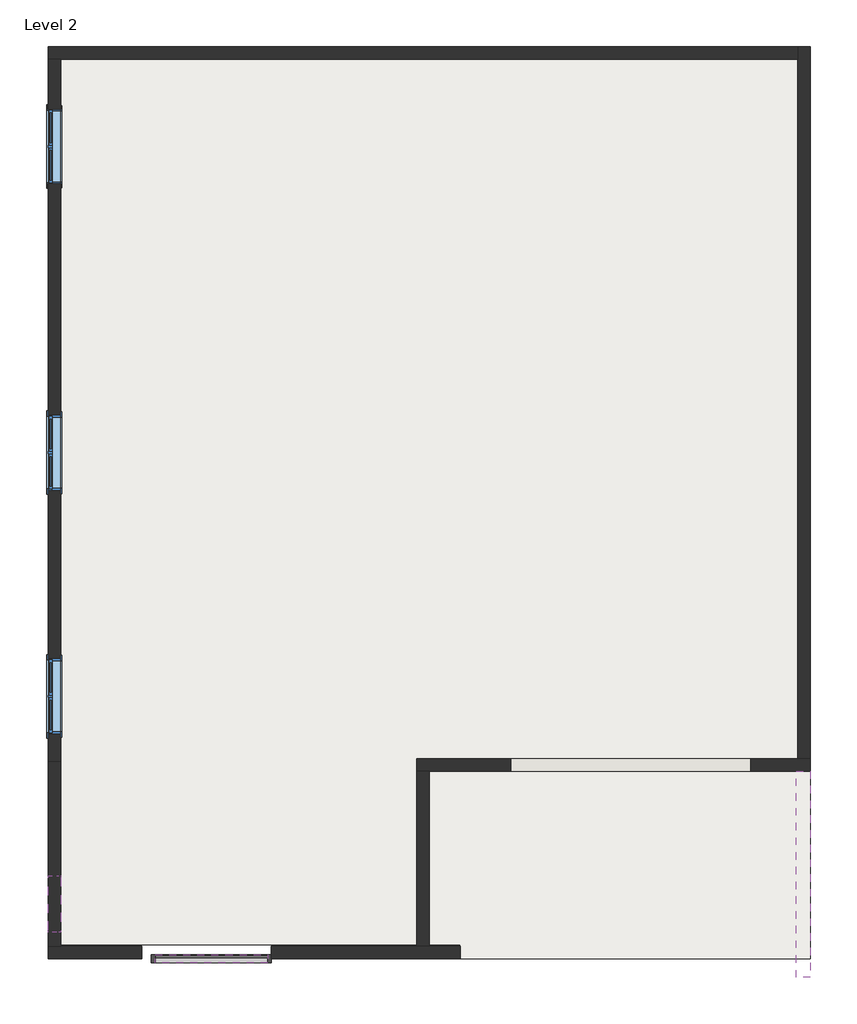
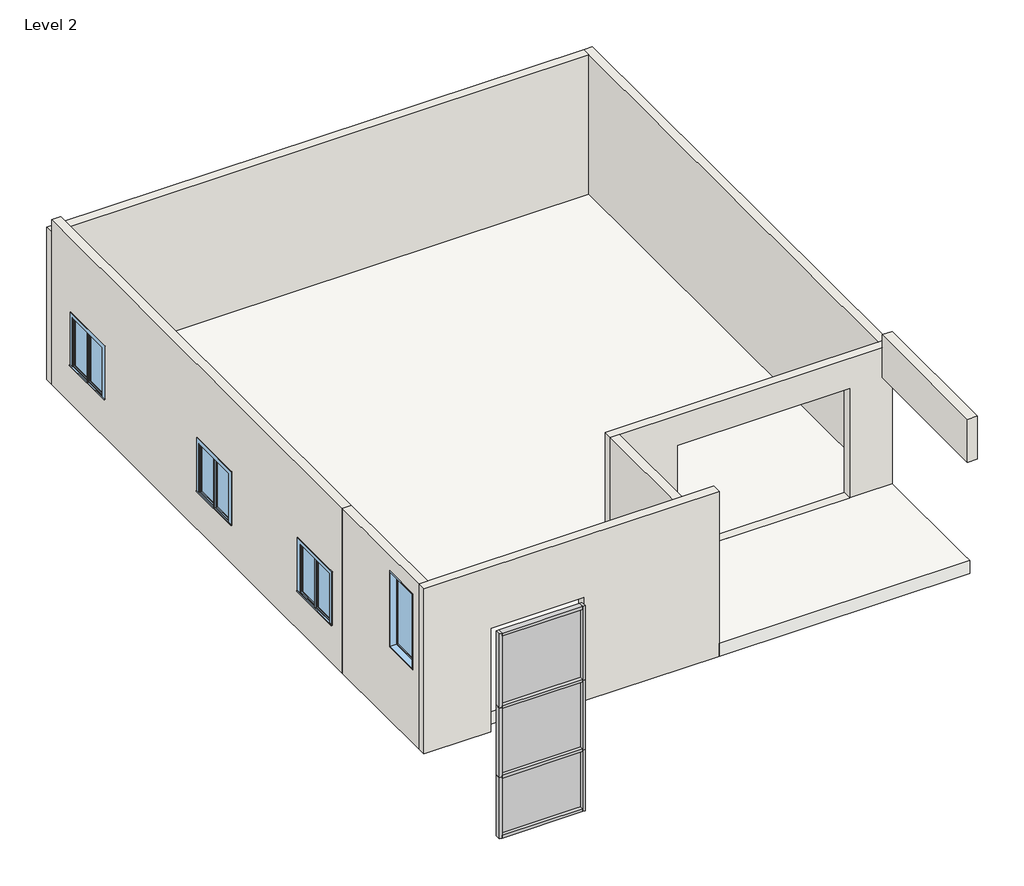
# One storey, incomplete: 10 members, 8 walls, 4 windows, 3 plates, 1 roof.
"""IFC4 building model written with IfcOpenShell, lengths in millimetres."""

from ifc_helpers import new_model, si_unit, frame, origin, place, context, project, spatial, polyline, outline, extrude, faceted_brep, transform, mapped, element, save
from components import member_75d123ff, member_e97ac6c9, member_a79ef8c7, member_78ce859c, member_f992ac7f, system_panel_glazed_7553f7e0, system_panel_glazed_3ebfe8c5, system_panel_glazed_c38f4616, walls_2_walls_2_0f297521, window_0862ab64, window_9a779fa2

model = new_model("IFC4")

# Units and contexts
model_context = context("Model", 3, world=origin())
ifc_project = project(units=[si_unit("LENGTHUNIT", "METRE", prefix="MILLI")], contexts=[model_context])

# Site, building, storey
site = spatial("IfcSite", under=ifc_project)
building = spatial("IfcBuilding", under=site)
storey = spatial("IfcBuildingStorey", under=building, Name="Level 2", Elevation=3657.6)

# Members
placement = place(None, origin())
member_shape = member_75d123ff(model_context)
element("IfcMember", 1, ObjectType="Rectangular Mullion : 2.5\" x 5\" rectangular", at=placement, inside=storey, context=model_context, shape_type="MappedRepresentation", body=[
    mapped(member_shape, transform((-4944.6813589, -4245.7139512, 2537.0926716), x_axis=(1.0, 0.0, 0.0), y_axis=(0.0, -1.0, 0.0), z_axis=(0.0, 0.0, -1.0))),
])
member_2_shape = member_e97ac6c9(model_context)
element("IfcMember", 2, ObjectType="Rectangular Mullion : 2.5\" x 5\" rectangular", at=placement, inside=storey, context=model_context, shape_type="MappedRepresentation", body=[
    mapped(member_2_shape, transform((-4944.6813589, -4245.7139512, 4210.5853432), x_axis=(1.0, 0.0, 0.0), y_axis=(0.0, -1.0, 0.0), z_axis=(0.0, 0.0, -1.0))),
])
member_3_shape = member_a79ef8c7(model_context)
element("IfcMember", 3, ObjectType="Rectangular Mullion : 2.5\" x 5\" rectangular", at=placement, inside=storey, context=model_context, shape_type="MappedRepresentation", body=[
    mapped(member_3_shape, transform((-4944.6813589, -4245.7139512, 1066.8), x_axis=(1.0, 0.0, 0.0), y_axis=(0.0, -1.0, 0.0), z_axis=(0.0, 0.0, -1.0))),
])
member_4_shape = member_78ce859c(model_context)
element("IfcMember", 4, ObjectType="Rectangular Mullion : 2.5\" x 5\" rectangular", at=placement, inside=storey, context=model_context, shape_type="MappedRepresentation", body=[
    mapped(member_4_shape, transform((-5008.1813589, -4245.7139512, 4210.5853432), x_axis=(0.0, 0.0, 1.0), y_axis=(0.0, -1.0, 0.0), z_axis=(1.0, 0.0, 0.0))),
])
element("IfcMember", 5, ObjectType="Rectangular Mullion : 2.5\" x 5\" rectangular", at=placement, inside=storey, context=model_context, shape_type="MappedRepresentation", body=[
    mapped(member_4_shape, transform((-5008.1813589, -4245.7139512, 2537.0926716), x_axis=(0.0, 0.0, 1.0), y_axis=(0.0, -1.0, 0.0), z_axis=(1.0, 0.0, 0.0))),
])
member_5_shape = member_f992ac7f(model_context)
element("IfcMember", 6, ObjectType="Rectangular Mullion : 2.5\" x 5\" rectangular", at=placement, inside=storey, context=model_context, shape_type="MappedRepresentation", body=[
    mapped(member_5_shape, transform((-5008.1813589, -4245.7139512, 5988.5853432), x_axis=(0.0, 0.0, 1.0), y_axis=(0.0, -1.0, 0.0), z_axis=(1.0, 0.0, 0.0))),
])
element("IfcMember", 7, ObjectType="Rectangular Mullion : 2.5\" x 5\" rectangular", at=placement, inside=storey, context=model_context, shape_type="MappedRepresentation", body=[
    mapped(member_5_shape, transform((-6833.2101057, -4245.7139512, 1066.8), x_axis=(0.0, 0.0, -1.0), y_axis=(0.0, -1.0, 0.0), z_axis=(-1.0, 0.0, 0.0))),
])
element("IfcMember", 8, ObjectType="Rectangular Mullion : 2.5\" x 5\" rectangular", at=placement, inside=storey, context=model_context, shape_type="MappedRepresentation", body=[
    mapped(member_3_shape, transform((-6896.7101057, -4245.7139512, 2537.0926716), x_axis=(-1.0, 0.0, 0.0), y_axis=(0.0, -1.0, 0.0), z_axis=(0.0, 0.0, 1.0))),
])
element("IfcMember", 9, ObjectType="Rectangular Mullion : 2.5\" x 5\" rectangular", at=placement, inside=storey, context=model_context, shape_type="MappedRepresentation", body=[
    mapped(member_shape, transform((-6896.7101057, -4245.7139512, 4210.5853432), x_axis=(-1.0, 0.0, 0.0), y_axis=(0.0, -1.0, 0.0), z_axis=(0.0, 0.0, 1.0))),
])
element("IfcMember", 10, ObjectType="Rectangular Mullion : 2.5\" x 5\" rectangular", at=placement, inside=storey, context=model_context, shape_type="MappedRepresentation", body=[
    mapped(member_2_shape, transform((-6896.7101057, -4245.7139512, 5988.5853432), x_axis=(-1.0, 0.0, 0.0), y_axis=(0.0, -1.0, 0.0), z_axis=(0.0, 0.0, 1.0))),
])

# Plates
system_panel_glazed_shape = system_panel_glazed_7553f7e0(model_context)
element("IfcPlate", 11, ObjectType="System Panel : Glazed", at=placement, inside=storey, context=model_context, shape_type="MappedRepresentation", body=[
    mapped(system_panel_glazed_shape, transform((-5920.6957323, -4245.7139512, 1130.3), x_axis=(1.0, 0.0, 0.0), y_axis=(0.0, 1.0, 0.0), z_axis=(0.0, 0.0, 1.0))),
])
system_panel_glazed_2_shape = system_panel_glazed_3ebfe8c5(model_context)
element("IfcPlate", 12, ObjectType="System Panel : Glazed", at=placement, inside=storey, context=model_context, shape_type="MappedRepresentation", body=[
    mapped(system_panel_glazed_2_shape, transform((-5920.6957323, -4245.7139512, 4242.3353432), x_axis=(1.0, 0.0, 0.0), y_axis=(0.0, 1.0, 0.0), z_axis=(0.0, 0.0, 1.0))),
])
system_panel_glazed_3_shape = system_panel_glazed_c38f4616(model_context)
element("IfcPlate", 13, ObjectType="System Panel : Glazed", at=placement, inside=storey, context=model_context, shape_type="MappedRepresentation", body=[
    mapped(system_panel_glazed_3_shape, transform((-5920.6957323, -4245.7139512, 2568.8426716), x_axis=(1.0, 0.0, 0.0), y_axis=(0.0, 1.0, 0.0), z_axis=(0.0, 0.0, 1.0))),
])

# Roof
element("IfcRoof", 14, ObjectType="Generic - 12\"", at=placement, inside=storey, context=model_context, shape_type="SweptSolid", body=[
    extrude(outline(polyline([(-8374.0311901, 10587.8860488), (3817.9688099, 10587.8860488), (3817.9688099, -4017.1139512), (3817.9688099, -4245.7139512), (-1871.6311901, -4245.7139512), (-1871.6311901, -4017.1139512), (-8374.0311901, -4017.1139512), (-8374.0311901, 10587.8860488)])), frame((0.0, 0.0, 3657.6), z_axis=(0.0, 0.0, 1.0), x_axis=(1.0, 0.0, 0.0)), (0.0, 0.0, 1.0), 304.8),
])

# Walls
element("IfcWall", 15, ObjectType="Generic - 8\"", at=placement, inside=storey, context=model_context, shape_type="Brep", body=[
    faceted_brep([(3817.9688099, -994.5139512, 3657.6), (3614.7688099, -994.5139512, 3657.6), (-2582.8311901, -994.5139512, 3657.6), (-2582.8311901, -994.5139512, 7315.2), (3614.7688099, -994.5139512, 7315.2), (3817.9688099, -994.5139512, 7315.2), (2852.2278443, -994.5139512, 6587.697392), (-1052.1762723, -994.5139512, 6587.697392), (-1052.1762723, -994.5139512, 3962.4), (2852.2278443, -994.5139512, 3962.4), (3817.9688099, -1197.7139512, 3657.6), (3817.9688099, -1197.7139512, 7315.2), (3589.3688099, -1197.7139512, 7315.2), (-2379.6311901, -1197.7139512, 7315.2), (-2582.8311901, -1197.7139512, 7315.2), (-2582.8311901, -1197.7139512, 3657.6), (-2379.6311901, -1197.7139512, 3657.6), (2852.2278443, -1197.7139512, 6587.697392), (2852.2278443, -1197.7139512, 3962.4), (-1052.1762723, -1197.7139512, 3962.4), (-1052.1762723, -1197.7139512, 6587.697392)], [[[0, 1, 2, 3, 4, 5], [6, 7, 8, 9]], [[10, 11, 12, 13, 14, 15, 16], [17, 18, 19, 20]], [[3, 2, 15, 14]], [[0, 5, 11, 10]], [[5, 4, 3, 14, 13, 12, 11]], [[2, 1, 0, 10, 16, 15]], [[7, 6, 17, 20]], [[8, 7, 20, 19]], [[9, 8, 19, 18]], [[6, 9, 18, 17]]]),
])
element("IfcWall", 16, ObjectType="Generic - 8\"", at=placement, inside=storey, context=model_context, shape_type="SweptSolid", body=[
    extrude(outline(polyline([(-1197.7139512, 3657.6), (-4042.5139512, 3657.6), (-4042.5139512, 7315.2), (-4017.1139512, 7315.2), (-1197.7139512, 7315.2), (-1197.7139512, 3657.6)])), frame((-2582.8311901, 0.0, 0.0), z_axis=(1.0, 0.0, 0.0), x_axis=(0.0, 1.0, 0.0)), (0.0, 0.0, 1.0), 203.2),
])
element("IfcWall", 17, ObjectType="Generic - 8\"", at=placement, inside=storey, context=model_context, shape_type="Brep", body=[
    faceted_brep([(3817.9688099, -994.5139512, 3657.6), (3817.9688099, 10587.8860488, 3657.6), (3817.9688099, 10587.8860488, 7315.2), (3817.9688099, -994.5139512, 7315.2), (3614.7688099, -994.5139512, 3657.6), (3614.7688099, -994.5139512, 7315.2), (3614.7688099, 10384.6860488, 7315.2), (3614.7688099, 10587.8860488, 7315.2), (3614.7688099, 10587.8860488, 3657.6), (3614.7688099, 10384.6860488, 3657.6)], [[[0, 1, 2, 3]], [[4, 5, 6, 7, 8, 9]], [[1, 0, 4, 9, 8]], [[0, 3, 5, 4]], [[2, 1, 8, 7]], [[3, 2, 7, 6, 5]]]),
])
element("IfcWall", 18, ObjectType="Generic - 8\"", at=placement, inside=storey, context=model_context, shape_type="Brep", body=[
    faceted_brep([(3614.7688099, 10587.8860488, 3657.6), (-8577.2311901, 10587.8860488, 3657.6), (-8577.2311901, 10587.8860488, 7315.2), (-8374.0311901, 10587.8860488, 7315.2), (3614.7688099, 10587.8860488, 7315.2), (3614.7688099, 10384.6860488, 3657.6), (3614.7688099, 10384.6860488, 7315.2), (-8374.0311901, 10384.6860488, 7315.2), (-8577.2311901, 10384.6860488, 7315.2), (-8577.2311901, 10384.6860488, 3657.6), (-8374.0311901, 10384.6860488, 3657.6)], [[[0, 1, 2, 3, 4]], [[5, 6, 7, 8, 9, 10]], [[1, 0, 5, 10, 9]], [[0, 4, 6, 5]], [[2, 1, 9, 8]], [[3, 2, 8, 7]], [[4, 3, 7, 6]]]),
])
element("IfcWall", 19, ObjectType="Generic - 8\"", at=placement, inside=storey, context=model_context, shape_type="Brep", body=[
    faceted_brep([(-8577.2311901, 10384.6860488, 3657.6), (-8577.2311901, -1045.3139512, 3657.6), (-8577.2311901, -1045.3139512, 7620.0), (-8577.2311901, 10384.6860488, 7620.0), (-8577.2311901, 10384.6860488, 7315.2), (-8577.2311901, 631.0860488, 5791.2), (-8577.2311901, -588.1139512, 5791.2), (-8577.2311901, -588.1139512, 4572.0), (-8577.2311901, 631.0860488, 4572.0), (-8577.2311901, 4593.4860488, 5791.2), (-8577.2311901, 3374.2860488, 5791.2), (-8577.2311901, 3374.2860488, 4572.0), (-8577.2311901, 4593.4860488, 4572.0), (-8577.2311901, 9571.8860488, 5791.2), (-8577.2311901, 8352.6860488, 5791.2), (-8577.2311901, 8352.6860488, 4572.0), (-8577.2311901, 9571.8860488, 4572.0), (-8374.0311901, 10384.6860488, 3657.6), (-8374.0311901, 10384.6860488, 7620.0), (-8374.0311901, -1045.3139512, 7620.0), (-8374.0311901, -1045.3139512, 3657.6), (-8374.0311901, 631.0860488, 5791.2), (-8374.0311901, 631.0860488, 4572.0), (-8374.0311901, -588.1139512, 4572.0), (-8374.0311901, -588.1139512, 5791.2), (-8374.0311901, 4593.4860488, 5791.2), (-8374.0311901, 4593.4860488, 4572.0), (-8374.0311901, 3374.2860488, 4572.0), (-8374.0311901, 3374.2860488, 5791.2), (-8374.0311901, 9571.8860488, 5791.2), (-8374.0311901, 9571.8860488, 4572.0), (-8374.0311901, 8352.6860488, 4572.0), (-8374.0311901, 8352.6860488, 5791.2)], [[[0, 1, 2, 3, 4], [5, 6, 7, 8], [9, 10, 11, 12], [13, 14, 15, 16]], [[17, 18, 19, 20], [21, 22, 23, 24], [25, 26, 27, 28], [29, 30, 31, 32]], [[1, 0, 17, 20]], [[2, 1, 20, 19]], [[3, 2, 19, 18]], [[0, 4, 3, 18, 17]], [[22, 21, 5, 8]], [[23, 22, 8, 7]], [[24, 23, 7, 6]], [[21, 24, 6, 5]], [[26, 25, 9, 12]], [[27, 26, 12, 11]], [[28, 27, 11, 10]], [[25, 28, 10, 9]], [[30, 29, 13, 16]], [[31, 30, 16, 15]], [[32, 31, 15, 14]], [[29, 32, 14, 13]]]),
])
element("IfcWall", 20, ObjectType="Generic - 8\"", at=placement, inside=storey, context=model_context, shape_type="Brep", body=[
    faceted_brep([(-8577.2311901, -4245.7139512, 7620.0), (-8577.2311901, -4245.7139512, 3657.6), (-8374.0311901, -4245.7139512, 3657.6), (-7057.7216902, -4245.7139512, 3657.6), (-7057.7216902, -4245.7139512, 6144.4106915), (-4944.6813589, -4245.7139512, 6144.4106915), (-4944.6813589, -4245.7139512, 3657.6), (-1871.6311901, -4245.7139512, 3657.6), (-1871.6311901, -4245.7139512, 7620.0), (-8374.0311901, -4245.7139512, 7620.0), (-8577.2311901, -4042.5139512, 3657.6), (-8577.2311901, -4042.5139512, 7620.0), (-8374.0311901, -4042.5139512, 7620.0), (-1871.6311901, -4042.5139512, 7620.0), (-1871.6311901, -4042.5139512, 3657.6), (-2379.6311901, -4042.5139512, 3657.6), (-2582.8311901, -4042.5139512, 3657.6), (-4944.6813589, -4042.5139512, 3657.6), (-4944.6813589, -4042.5139512, 6144.4106915), (-7057.7216902, -4042.5139512, 6144.4106915), (-7057.7216902, -4042.5139512, 3657.6), (-8374.0311901, -4042.5139512, 3657.6)], [[[0, 1, 2, 3, 4, 5, 6, 7, 8, 9]], [[10, 11, 12, 13, 14, 15, 16, 17, 18, 19, 20, 21]], [[0, 11, 10, 1]], [[8, 7, 14, 13]], [[0, 9, 8, 13, 12, 11]], [[3, 2, 1, 10, 21, 20]], [[4, 3, 20, 19]], [[5, 4, 19, 18]], [[6, 5, 18, 17]], [[7, 6, 17, 16, 15, 14]]]),
])
element("IfcWall", 21, ObjectType="Generic - 8\"", at=placement, inside=storey, context=model_context, shape_type="SweptSolid", body=[
    extrude(outline(polyline([(-1045.3139512, 3657.6), (-4042.5139512, 3657.6), (-4042.5139512, 7620.0), (-1045.3139512, 7620.0), (-1045.3139512, 3657.6)]), holes=[polyline([(-3813.9139512, 7245.9057728), (-3813.9139512, 5417.1057728), (-2899.5139512, 5417.1057728), (-2899.5139512, 7245.9057728), (-3813.9139512, 7245.9057728)])]), frame((-8577.2311901, 0.0, 0.0), z_axis=(1.0, 0.0, 0.0), x_axis=(0.0, 1.0, 0.0)), (0.0, 0.0, 1.0), 203.2),
])
walls_2_walls_2_shape = walls_2_walls_2_0f297521(model_context)
element("IfcWall", 22, ObjectType="Walls 2 : Walls 2", at=placement, inside=storey, context=model_context, shape_type="MappedRepresentation", body=[
    mapped(walls_2_walls_2_shape, transform((0.0, 0.0, 0.0), x_axis=(1.0, 0.0, 0.0), y_axis=(0.0, 1.0, 0.0), z_axis=(0.0, 0.0, 1.0))),
])

# Windows
window_shape = window_0862ab64(model_context)
element("IfcWindow", 23, ObjectType="Casement Dbl with Trim : 48\" x 48\"", at=placement, inside=storey, context=model_context, shape_type="MappedRepresentation", body=[
    mapped(window_shape, transform((-8456.5811901, 21.4860488, 3657.6), x_axis=(0.0, 1.0, 0.0), y_axis=(-1.0, 0.0, 0.0), z_axis=(0.0, 0.0, 1.0))),
])
element("IfcWindow", 24, ObjectType="Casement Dbl with Trim : 48\" x 48\"", at=placement, inside=storey, context=model_context, shape_type="MappedRepresentation", body=[
    mapped(window_shape, transform((-8456.5811901, 3983.8860488, 3657.6), x_axis=(0.0, 1.0, 0.0), y_axis=(-1.0, 0.0, 0.0), z_axis=(0.0, 0.0, 1.0))),
])
element("IfcWindow", 25, ObjectType="Casement Dbl with Trim : 48\" x 48\"", at=placement, inside=storey, context=model_context, shape_type="MappedRepresentation", body=[
    mapped(window_shape, transform((-8456.5811901, 8962.2860488, 3657.6), x_axis=(0.0, 1.0, 0.0), y_axis=(-1.0, 0.0, 0.0), z_axis=(0.0, 0.0, 1.0))),
])
window_2_shape = window_9a779fa2(model_context)
element("IfcWindow", 26, ObjectType="Fixed : 36\" x 72\"", at=placement, inside=storey, context=model_context, shape_type="MappedRepresentation", body=[
    mapped(window_2_shape, transform((-8475.6311901, -3394.8139512, 5112.3057728), x_axis=(0.0, -1.0, 0.0), y_axis=(1.0, 0.0, 0.0), z_axis=(0.0, 0.0, 1.0))),
])

save(model, "model.ifc")

# Revit data of these elements
# Type "Rectangular Mullion : 2.5\" x 5\" rectangular"
#   built-in parameter 1007304 = 0.416667 (stored number, unit not read)
#   built-in parameter 1007301 = 0.104167 (stored number, unit not read)
#   built-in parameter 1007300 = 0.104167 (stored number, unit not read)
# Type "System Panel : Glazed"
#   Construction Type Id = "GSP4R"
#   Analytic Construction = "1/8 in Pilkington single glazing"
#   Visual Light Transmittance = 0.9
#   Solar Heat Gain Coefficient = 0.86
#   Heat Transfer Coefficient (U) = 1.18115 BTU/(h·ft²·°F)
# Type "Generic - 12\""
#   Assembly Code = "B1020"
#   Layers, outside or top first: 1' - 0" no material (function 1)
# Type "Generic - 8\""
#   Assembly Code = "B2010"
#   Layers, outside or top first: 0' - 8" no material (function 1)
# Type "Casement Dbl with Trim : 48\" x 48\""
#   Type Mark = "10"
#   Construction Type Id = "GSP4R"
#   Assembly Code = "B2020100"
#   Analytic Construction = "1/8 in Pilkington single glazing"
#   Visual Light Transmittance = 0.9
#   Thermal Resistance (R) = 1.53941 (h·ft²·°F)/BTU
#   Solar Heat Gain Coefficient = 0.78
#   Heat Transfer Coefficient (U) = 0.6496 BTU/(h·ft²·°F)
#   Height = 4' - 0"
#   Default Sill Height = 3' - 0"
#   Trim Projection - Ext. = 0' - 0 1/2"
#   Trim Projection - Int. = 0' - 0 3/4"
#   Trim Width - Exterior = 0' - 3 1/2"
#   Trim Width - Interior = 0' - 3 1/2"
#   Width = 4' - 0"
#   Window Inset = 0' - 0 3/4"
#   Define Thermal Properties by = 1
#   Glass Pane Material = Glass
#   Sash Material = Sash
#   Trim Exterior Material = Trim
#   Trim Interior Material = Trim
#   Wall Closure = (empty or 0)
# Type "Fixed : 36\" x 72\""
#   Type Mark = "9"
#   Construction Type Id = "GSP4R"
#   Assembly Code = "B2020100"
#   Analytic Construction = "1/8 in Pilkington single glazing"
#   Visual Light Transmittance = 0.9
#   Solar Heat Gain Coefficient = 0.78
#   Heat Transfer Coefficient (U) = 0.6496 BTU/(h·ft²·°F)
#   Height = 6' - 0"
#   Default Sill Height = 1' - 0"
#   Width = 3' - 0"
#   Window Inset = 0' - 0 3/4"
#   Define Thermal Properties by = 1
#   Glass Pane Material = Glass
#   Sash Material = Sash
#   Wall Closure = (empty or 0)
# Elements 1, 2, 3, 4, 5, 6, 7, 8, 9, 10 (IfcMember, "Rectangular Mullion : 2.5\" x 5\" rectangular")
#   Phase Created = New Construction
#   Materials on its faces: "Aluminum"
# Elements 11, 12, 13 (IfcPlate, "System Panel : Glazed")
#   Phase Created = New Construction
#   Materials on its faces: "Glass"
# Element 14 (IfcRoof, "Generic - 12\"")
#   built-in parameter 1001705 = 13 (stored number, unit not read)
#   built-in parameter 1001710 = 33615
#   Phase Created = New Construction
#   Materials on its faces: "Default Roof"
# Elements 15, 16, 17, 18 (IfcWall, "Generic - 8\"")
#   Top Offset = 0' - 0"
#   Base Offset = 0' - 0"
#   Unconnected Height = 12' - 0"
#   wall height = 12' - 0"
#   Phase Created = New Construction
#   Base Constraint = Level 2
#   Materials on its faces: "Default Wall"
# Elements 19, 20, 21 (IfcWall, "Generic - 8\"")
#   Top Offset = 0' - 0"
#   Base Offset = 0' - 0"
#   Unconnected Height = 13' - 0"
#   wall height = 13' - 0"
#   Phase Created = New Construction
#   Base Constraint = Level 2
#   Materials on its faces: "Default Wall"
# Element 22 (IfcWall, "Walls 2 : Walls 2")
#   Phase Created = New Construction
#   Materials on its faces: "Default Wall"
# Element 23 (IfcWindow, "Casement Dbl with Trim : 48\" x 48\"")
#   Mark = "3"
#   Phase Created = New Construction
#   Materials on its faces: "Sash", "Trim", "Glass"
# Element 24 (IfcWindow, "Casement Dbl with Trim : 48\" x 48\"")
#   Mark = "4"
#   Phase Created = New Construction
#   Materials on its faces: "Sash", "Trim", "Glass"
# Element 25 (IfcWindow, "Casement Dbl with Trim : 48\" x 48\"")
#   Mark = "5"
#   Phase Created = New Construction
#   Materials on its faces: "Sash", "Trim", "Glass"
# Element 26 (IfcWindow, "Fixed : 36\" x 72\"")
#   Mark = "1"
#   Phase Created = New Construction
#   Materials on its faces: "Sash", "Glass"
# Materials
#   "Glass": class "Glass", colour RGB 0 128 192, transparency 0.75, Description = "Soda Lime Glass", Cost = 0
#   "Sash": class "Wood", colour RGB 224 178 126, transparency 0
#   "Trim": class "Wood", colour RGB 224 178 126, transparency 0
#   "Aluminum": class "Metal", colour RGB 247 247 247, transparency 0, Description = "Aluminum 6061", Cost = 0
#   "Default Roof": colour RGB 88 101 114, transparency 0
#   "Default Wall": colour RGB 128 128 128, transparency 0
